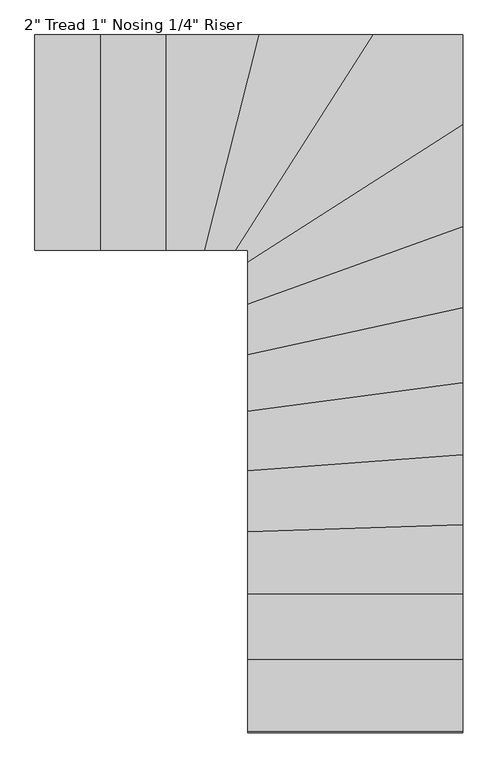
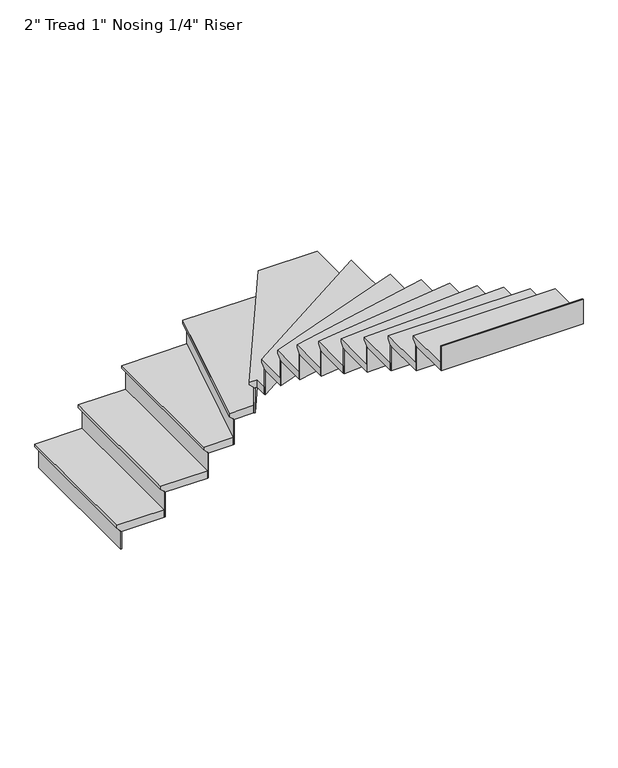
"""IFC4 building model written with IfcOpenShell, lengths in millimetres: stair flight geometry."""

from ifc_helpers import new_model, si_unit, origin, place, context, project, spatial, faceted_brep, source, transform, mapped, element, save


def stair_flight_d6903057(model_context):
    return source(origin(), model_context, "Body", "Brep", [
        faceted_brep([(-12520.2436952, 5104.5187882, 827.6166667), (-12520.2436952, 5104.5187882, 846.6666667), (-12520.2436952, 6018.9187882, 846.6666667), (-12520.2436952, 6018.9187882, 827.6166667), (-12494.8436952, 5104.5187882, 802.2166667), (-12494.8436952, 6018.9187882, 802.2166667), (-12215.4436952, 5104.5187882, 846.6666667), (-12215.4436952, 6018.9187882, 846.6666667), (-12494.8436952, 6018.9187882, 795.8666667), (-12215.4436952, 6018.9187882, 795.8666667), (-12215.4436952, 5104.5187882, 795.8666667), (-12494.8436952, 5104.5187882, 795.8666667)], [[[0, 1, 2, 3]], [[4, 0, 3, 5]], [[2, 1, 6, 7]], [[8, 9, 10, 11]], [[2, 7, 9, 8, 5, 3]], [[8, 11, 4, 5]], [[6, 1, 0, 4, 11, 10]], [[7, 6, 10, 9]]]),
        faceted_brep([(-12494.8436952, 5104.5187882, 795.8666667), (-12494.8436952, 5104.5187882, 677.3333333), (-12488.4936952, 5104.5187882, 677.3333333), (-12488.4936952, 5104.5187882, 795.8666667), (-12494.8436952, 6018.9187882, 795.8666667), (-12488.4936952, 6018.9187882, 795.8666667), (-12488.4936952, 6018.9187882, 677.3333333), (-12494.8436952, 6018.9187882, 677.3333333)], [[[0, 1, 2, 3]], [[4, 5, 6, 7]], [[1, 0, 4, 7]], [[2, 1, 7, 6]], [[3, 2, 6, 5]], [[0, 3, 5, 4]]]),
        faceted_brep([(-12215.4436952, 5104.5187882, 965.2), (-12215.4436952, 5104.5187882, 795.8666667), (-12209.0936952, 5104.5187882, 795.8666667), (-12209.0936952, 5104.5187882, 965.2), (-12215.4436952, 6018.9187882, 965.2), (-12209.0936952, 6018.9187882, 965.2), (-12209.0936952, 6018.9187882, 795.8666667), (-12215.4436952, 6018.9187882, 795.8666667)], [[[0, 1, 2, 3]], [[4, 5, 6, 7]], [[1, 0, 4, 7]], [[2, 1, 7, 6]], [[3, 2, 6, 5]], [[0, 3, 5, 4]]]),
        faceted_brep([(-12240.8436952, 6018.9187882, 1016.0), (-12240.8436952, 5104.5187882, 1016.0), (-11936.0436952, 5104.5187882, 1016.0), (-11936.0436952, 6018.9187882, 1016.0), (-12215.4436952, 6018.9187882, 965.2), (-11936.0436952, 6018.9187882, 965.2), (-11936.0436952, 5104.5187882, 965.2), (-12215.4436952, 5104.5187882, 965.2), (-12215.4436952, 6018.9187882, 971.55), (-12240.8436952, 6018.9187882, 996.95), (-12215.4436952, 5104.5187882, 971.55), (-12240.8436952, 5104.5187882, 996.95)], [[[0, 1, 2, 3]], [[4, 5, 6, 7]], [[0, 3, 5, 4, 8, 9]], [[4, 7, 10, 8]], [[2, 1, 11, 10, 7, 6]], [[3, 2, 6, 5]], [[11, 1, 0, 9]], [[10, 11, 9, 8]]]),
        faceted_brep([(-11936.0436952, 5104.5187882, 1134.5333333), (-11936.0436952, 5104.5187882, 965.2), (-11929.6936952, 5104.5187882, 965.2), (-11929.6936952, 5104.5187882, 1134.5333333), (-11936.0436952, 6018.9187882, 1134.5333333), (-11929.6936952, 6018.9187882, 1134.5333333), (-11929.6936952, 6018.9187882, 965.2), (-11936.0436952, 6018.9187882, 965.2)], [[[0, 1, 2, 3]], [[4, 5, 6, 7]], [[1, 0, 4, 7]], [[2, 1, 7, 6]], [[3, 2, 6, 5]], [[0, 3, 5, 4]]]),
        faceted_brep([(-11961.4436952, 6018.9187882, 1185.3333333), (-11961.4436952, 5104.5187882, 1185.3333333), (-11771.3386614, 5104.5187882, 1185.3333333), (-11540.3529848, 6018.9187882, 1185.3333333), (-11936.0436952, 6018.9187882, 1134.5333333), (-11540.3529848, 6018.9187882, 1134.5333333), (-11771.3386614, 5104.5187882, 1134.5333333), (-11936.0436952, 5104.5187882, 1134.5333333), (-11936.0436952, 6018.9187882, 1140.8833333), (-11961.4436952, 6018.9187882, 1166.2833333), (-11936.0436952, 5104.5187882, 1140.8833333), (-11961.4436952, 5104.5187882, 1166.2833333)], [[[0, 1, 2, 3]], [[4, 5, 6, 7]], [[0, 3, 5, 4, 8, 9]], [[4, 7, 10, 8]], [[2, 1, 11, 10, 7, 6]], [[3, 2, 6, 5]], [[11, 1, 0, 9]], [[10, 11, 9, 8]]]),
        faceted_brep([(-11771.3386614, 5104.5187882, 1303.8666667), (-11771.3386614, 5104.5187882, 1134.5333333), (-11764.7891933, 5104.5187882, 1134.5333333), (-11764.7891933, 5104.5187882, 1303.8666667), (-11540.3529848, 6018.9187882, 1303.8666667), (-11533.8035167, 6018.9187882, 1303.8666667), (-11533.8035167, 6018.9187882, 1134.5333333), (-11540.3529848, 6018.9187882, 1134.5333333)], [[[0, 1, 2, 3]], [[4, 5, 6, 7]], [[1, 0, 4, 7]], [[2, 1, 7, 6]], [[3, 2, 6, 5]], [[0, 3, 5, 4]]]),
        faceted_brep([(-11566.5508569, 6018.9187882, 1354.6666667), (-11797.5365335, 5104.5187882, 1354.6666667), (-11637.0710723, 5104.5187882, 1354.6666667), (-11052.4716369, 6018.9187882, 1354.6666667), (-11540.3529848, 6018.9187882, 1303.8666667), (-11052.4716369, 6018.9187882, 1303.8666667), (-11637.0710723, 5104.5187882, 1303.8666667), (-11771.3386614, 5104.5187882, 1303.8666667), (-11540.3529848, 6018.9187882, 1310.2166667), (-11566.5508569, 6018.9187882, 1335.6166667), (-11771.3386614, 5104.5187882, 1310.2166667), (-11797.5365335, 5104.5187882, 1335.6166667)], [[[0, 1, 2, 3]], [[4, 5, 6, 7]], [[0, 3, 5, 4, 8, 9]], [[4, 7, 10, 8]], [[2, 1, 11, 10, 7, 6]], [[3, 2, 6, 5]], [[11, 1, 0, 9]], [[10, 11, 9, 8]]]),
        faceted_brep([(-11637.0710723, 5104.5187882, 1473.2), (-11637.0710723, 5104.5187882, 1303.8666667), (-11629.5342419, 5104.5187882, 1303.8666667), (-11629.5342419, 5104.5187882, 1473.2), (-11052.4716369, 6018.9187882, 1473.2), (-11044.9348065, 6018.9187882, 1473.2), (-11044.9348065, 6018.9187882, 1303.8666667), (-11052.4716369, 6018.9187882, 1303.8666667)], [[[0, 1, 2, 3]], [[4, 5, 6, 7]], [[1, 0, 4, 7]], [[2, 1, 7, 6]], [[3, 2, 6, 5]], [[0, 3, 5, 4]]]),
        faceted_brep([(-10701.9067057, 5608.0592137, 1524.0), (-10701.9067057, 6018.9187882, 1524.0), (-11082.6189586, 6018.9187882, 1524.0), (-11667.218394, 5104.5187882, 1524.0), (-11616.3067057, 5104.5187882, 1524.0), (-11616.3067057, 5023.4597783, 1524.0), (-10701.9067057, 6018.9187882, 1473.2), (-10701.9067057, 5608.0592137, 1473.2), (-11616.3067057, 5023.4597783, 1473.2), (-11616.3067057, 5104.5187882, 1473.2), (-11637.0710723, 5104.5187882, 1473.2), (-11052.4716369, 6018.9187882, 1473.2), (-11637.0710723, 5104.5187882, 1479.55), (-11052.4716369, 6018.9187882, 1479.55), (-11667.218394, 5104.5187882, 1504.95), (-11082.6189586, 6018.9187882, 1504.95)], [[[0, 1, 2, 3, 4, 5]], [[6, 7, 8, 9, 10, 11]], [[1, 0, 7, 6]], [[11, 10, 12, 13]], [[4, 3, 14, 12, 10, 9]], [[0, 5, 8, 7]], [[14, 3, 2, 15]], [[12, 14, 15, 13]], [[2, 1, 6, 11, 13, 15]], [[5, 4, 9, 8]]]),
        faceted_brep([(-11616.3067057, 5023.4597783, 1642.5333333), (-11616.3067057, 5023.4597783, 1473.2), (-11616.3067057, 5015.9229479, 1473.2), (-11616.3067057, 5015.9229479, 1642.5333333), (-10701.9067057, 5608.0592137, 1642.5333333), (-10701.9067057, 5600.5223833, 1642.5333333), (-10701.9067057, 5600.5223833, 1473.2), (-10701.9067057, 5608.0592137, 1473.2)], [[[0, 1, 2, 3]], [[4, 5, 6, 7]], [[1, 0, 4, 7]], [[2, 1, 7, 6]], [[3, 2, 6, 5]], [[0, 3, 5, 4]]]),
        faceted_brep([(-10701.9067057, 5638.2065353, 1693.3333333), (-11616.3067057, 5053.6070999, 1693.3333333), (-11616.3067057, 4847.5034664, 1693.3333333), (-10701.9067057, 5176.0799712, 1693.3333333), (-10701.9067057, 5608.0592137, 1642.5333333), (-10701.9067057, 5176.0799712, 1642.5333333), (-11616.3067057, 4847.5034664, 1642.5333333), (-11616.3067057, 5023.4597783, 1642.5333333), (-10701.9067057, 5608.0592137, 1648.8833333), (-10701.9067057, 5638.2065353, 1674.2833333), (-11616.3067057, 5023.4597783, 1648.8833333), (-11616.3067057, 5053.6070999, 1674.2833333)], [[[0, 1, 2, 3]], [[4, 5, 6, 7]], [[0, 3, 5, 4, 8, 9]], [[4, 7, 10, 8]], [[2, 1, 11, 10, 7, 6]], [[3, 2, 6, 5]], [[11, 1, 0, 9]], [[10, 11, 9, 8]]]),
        faceted_brep([(-11616.3067057, 4847.5034664, 1811.8666667), (-11616.3067057, 4847.5034664, 1642.5333333), (-11616.3067057, 4840.7559464, 1642.5333333), (-11616.3067057, 4840.7559464, 1811.8666667), (-10701.9067057, 5176.0799712, 1811.8666667), (-10701.9067057, 5169.3324512, 1811.8666667), (-10701.9067057, 5169.3324512, 1642.5333333), (-10701.9067057, 5176.0799712, 1642.5333333)], [[[0, 1, 2, 3]], [[4, 5, 6, 7]], [[1, 0, 4, 7]], [[2, 1, 7, 6]], [[3, 2, 6, 5]], [[0, 3, 5, 4]]]),
        faceted_brep([(-10701.9067057, 5203.0700511, 1862.6666667), (-11616.3067057, 4874.4935463, 1862.6666667), (-11616.3067057, 4633.3870673, 1862.6666667), (-10701.9067057, 4833.3757339, 1862.6666667), (-10701.9067057, 5176.0799712, 1811.8666667), (-10701.9067057, 4833.3757339, 1811.8666667), (-11616.3067057, 4633.3870673, 1811.8666667), (-11616.3067057, 4847.5034664, 1811.8666667), (-10701.9067057, 5176.0799712, 1818.2166667), (-10701.9067057, 5203.0700511, 1843.6166667), (-11616.3067057, 4847.5034664, 1818.2166667), (-11616.3067057, 4874.4935463, 1843.6166667)], [[[0, 1, 2, 3]], [[4, 5, 6, 7]], [[0, 3, 5, 4, 8, 9]], [[4, 7, 10, 8]], [[2, 1, 11, 10, 7, 6]], [[3, 2, 6, 5]], [[11, 1, 0, 9]], [[10, 11, 9, 8]]]),
        faceted_brep([(-11616.3067057, 4633.3870673, 1981.2), (-11616.3067057, 4633.3870673, 1811.8666667), (-11616.3067057, 4626.8869678, 1811.8666667), (-11616.3067057, 4626.8869678, 1981.2), (-10701.9067057, 4833.3757339, 1981.2), (-10701.9067057, 4826.8756344, 1981.2), (-10701.9067057, 4826.8756344, 1811.8666667), (-10701.9067057, 4833.3757339, 1811.8666667)], [[[0, 1, 2, 3]], [[4, 5, 6, 7]], [[1, 0, 4, 7]], [[2, 1, 7, 6]], [[3, 2, 6, 5]], [[0, 3, 5, 4]]]),
        faceted_brep([(-10701.9067057, 4859.376132, 2032.0), (-11616.3067057, 4659.3874654, 2032.0), (-11616.3067057, 4393.8400272, 2032.0), (-10701.9067057, 4514.8804393, 2032.0), (-10701.9067057, 4833.3757339, 1981.2), (-10701.9067057, 4514.8804393, 1981.2), (-11616.3067057, 4393.8400272, 1981.2), (-11616.3067057, 4633.3870673, 1981.2), (-10701.9067057, 4833.3757339, 1987.55), (-10701.9067057, 4859.376132, 2012.95), (-11616.3067057, 4633.3870673, 1987.55), (-11616.3067057, 4659.3874654, 2012.95)], [[[0, 1, 2, 3]], [[4, 5, 6, 7]], [[0, 3, 5, 4, 8, 9]], [[4, 7, 10, 8]], [[2, 1, 11, 10, 7, 6]], [[3, 2, 6, 5]], [[11, 1, 0, 9]], [[10, 11, 9, 8]]]),
        faceted_brep([(-11616.3067057, 4393.8400272, 2150.5333333), (-11616.3067057, 4393.8400272, 1981.2), (-11616.3067057, 4387.4346359, 1981.2), (-11616.3067057, 4387.4346359, 2150.5333333), (-10701.9067057, 4514.8804393, 2150.5333333), (-10701.9067057, 4508.4750479, 2150.5333333), (-10701.9067057, 4508.4750479, 1981.2), (-10701.9067057, 4514.8804393, 1981.2)], [[[0, 1, 2, 3]], [[4, 5, 6, 7]], [[1, 0, 4, 7]], [[2, 1, 7, 6]], [[3, 2, 6, 5]], [[0, 3, 5, 4]]]),
        faceted_brep([(-10701.9067057, 4540.5020047, 2201.3333333), (-11616.3067057, 4419.4615927, 2201.3333333), (-11616.3067057, 4141.2933024, 2201.3333333), (-10701.9067057, 4208.9315067, 2201.3333333), (-10701.9067057, 4514.8804393, 2150.5333333), (-10701.9067057, 4208.9315067, 2150.5333333), (-11616.3067057, 4141.2933024, 2150.5333333), (-11616.3067057, 4393.8400272, 2150.5333333), (-10701.9067057, 4514.8804393, 2156.8833333), (-10701.9067057, 4540.5020047, 2182.2833333), (-11616.3067057, 4393.8400272, 2156.8833333), (-11616.3067057, 4419.4615927, 2182.2833333)], [[[0, 1, 2, 3]], [[4, 5, 6, 7]], [[0, 3, 5, 4, 8, 9]], [[4, 7, 10, 8]], [[2, 1, 11, 10, 7, 6]], [[3, 2, 6, 5]], [[11, 1, 0, 9]], [[10, 11, 9, 8]]]),
        faceted_brep([(-11616.3067057, 4141.2933024, 2319.8666667), (-11616.3067057, 4141.2933024, 2150.5333333), (-11616.3067057, 4134.9259539, 2150.5333333), (-11616.3067057, 4134.9259539, 2319.8666667), (-10701.9067057, 4208.9315067, 2319.8666667), (-10701.9067057, 4202.5641582, 2319.8666667), (-10701.9067057, 4202.5641582, 2150.5333333), (-10701.9067057, 4208.9315067, 2150.5333333)], [[[0, 1, 2, 3]], [[4, 5, 6, 7]], [[1, 0, 4, 7]], [[2, 1, 7, 6]], [[3, 2, 6, 5]], [[0, 3, 5, 4]]]),
        faceted_brep([(-10701.9067057, 4234.4009008, 2370.6666667), (-11616.3067057, 4166.7626966, 2370.6666667), (-11616.3067057, 3881.2141892, 2370.6666667), (-10701.9067057, 3910.3236734, 2370.6666667), (-10701.9067057, 4208.9315067, 2319.8666667), (-10701.9067057, 3910.3236734, 2319.8666667), (-11616.3067057, 3881.2141892, 2319.8666667), (-11616.3067057, 4141.2933024, 2319.8666667), (-10701.9067057, 4208.9315067, 2326.2166667), (-10701.9067057, 4234.4009008, 2351.6166667), (-11616.3067057, 4141.2933024, 2326.2166667), (-11616.3067057, 4166.7626966, 2351.6166667)], [[[0, 1, 2, 3]], [[4, 5, 6, 7]], [[0, 3, 5, 4, 8, 9]], [[4, 7, 10, 8]], [[2, 1, 11, 10, 7, 6]], [[3, 2, 6, 5]], [[11, 1, 0, 9]], [[10, 11, 9, 8]]]),
        faceted_brep([(-11616.3067057, 3881.2141892, 2489.2), (-11616.3067057, 3881.2141892, 2319.8666667), (-11616.3067057, 3874.8609724, 2319.8666667), (-11616.3067057, 3874.8609724, 2489.2), (-10701.9067057, 3910.3236734, 2489.2), (-10701.9067057, 3903.9704565, 2489.2), (-10701.9067057, 3903.9704565, 2319.8666667), (-10701.9067057, 3910.3236734, 2319.8666667)], [[[0, 1, 2, 3]], [[4, 5, 6, 7]], [[1, 0, 4, 7]], [[2, 1, 7, 6]], [[3, 2, 6, 5]], [[0, 3, 5, 4]]]),
        faceted_brep([(-10701.9067057, 3935.7365407, 2540.0), (-11616.3067057, 3906.6270566, 2540.0), (-11616.3067057, 3616.3817987, 2540.0), (-10701.9067057, 3616.3817987, 2540.0), (-10701.9067057, 3910.3236734, 2489.2), (-10701.9067057, 3616.3817987, 2489.2), (-11616.3067057, 3616.3817987, 2489.2), (-11616.3067057, 3881.2141892, 2489.2), (-10701.9067057, 3910.3236734, 2495.55), (-10701.9067057, 3935.7365407, 2520.95), (-11616.3067057, 3881.2141892, 2495.55), (-11616.3067057, 3906.6270566, 2520.95)], [[[0, 1, 2, 3]], [[4, 5, 6, 7]], [[0, 3, 5, 4, 8, 9]], [[4, 7, 10, 8]], [[2, 1, 11, 10, 7, 6]], [[3, 2, 6, 5]], [[11, 1, 0, 9]], [[10, 11, 9, 8]]]),
        faceted_brep([(-11616.3067057, 3616.3817987, 2658.5333333), (-11616.3067057, 3616.3817987, 2489.2), (-11616.3067057, 3610.0317987, 2489.2), (-11616.3067057, 3610.0317987, 2658.5333333), (-10701.9067057, 3616.3817987, 2658.5333333), (-10701.9067057, 3610.0317987, 2658.5333333), (-10701.9067057, 3610.0317987, 2489.2), (-10701.9067057, 3616.3817987, 2489.2)], [[[0, 1, 2, 3]], [[4, 5, 6, 7]], [[1, 0, 4, 7]], [[2, 1, 7, 6]], [[3, 2, 6, 5]], [[0, 3, 5, 4]]]),
        faceted_brep([(-10701.9067057, 3641.7817987, 2709.3333333), (-11616.3067057, 3641.7817987, 2709.3333333), (-11616.3067057, 3336.9817987, 2709.3333333), (-10701.9067057, 3336.9817987, 2709.3333333), (-10701.9067057, 3616.3817987, 2658.5333333), (-10701.9067057, 3336.9817987, 2658.5333333), (-11616.3067057, 3336.9817987, 2658.5333333), (-11616.3067057, 3616.3817987, 2658.5333333), (-10701.9067057, 3616.3817987, 2664.8833333), (-10701.9067057, 3641.7817987, 2690.2833333), (-11616.3067057, 3616.3817987, 2664.8833333), (-11616.3067057, 3641.7817987, 2690.2833333)], [[[0, 1, 2, 3]], [[4, 5, 6, 7]], [[0, 3, 5, 4, 8, 9]], [[4, 7, 10, 8]], [[2, 1, 11, 10, 7, 6]], [[3, 2, 6, 5]], [[11, 1, 0, 9]], [[10, 11, 9, 8]]]),
        faceted_brep([(-11616.3067057, 3336.9817987, 2827.8666667), (-11616.3067057, 3336.9817987, 2658.5333333), (-11616.3067057, 3330.6317987, 2658.5333333), (-11616.3067057, 3330.6317987, 2827.8666667), (-10701.9067057, 3336.9817987, 2827.8666667), (-10701.9067057, 3330.6317987, 2827.8666667), (-10701.9067057, 3330.6317987, 2658.5333333), (-10701.9067057, 3336.9817987, 2658.5333333)], [[[0, 1, 2, 3]], [[4, 5, 6, 7]], [[1, 0, 4, 7]], [[2, 1, 7, 6]], [[3, 2, 6, 5]], [[0, 3, 5, 4]]]),
        faceted_brep([(-11616.3067057, 3057.5817987, 2997.2), (-11616.3067057, 3057.5817987, 2827.8666667), (-11616.3067057, 3051.2317987, 2827.8666667), (-11616.3067057, 3051.2317987, 2997.2), (-10701.9067057, 3057.5817987, 2997.2), (-10701.9067057, 3051.2317987, 2997.2), (-10701.9067057, 3051.2317987, 2827.8666667), (-10701.9067057, 3057.5817987, 2827.8666667)], [[[0, 1, 2, 3]], [[4, 5, 6, 7]], [[1, 0, 4, 7]], [[2, 1, 7, 6]], [[3, 2, 6, 5]], [[0, 3, 5, 4]]]),
        faceted_brep([(-10701.9067057, 3362.3817987, 2878.6666667), (-11616.3067057, 3362.3817987, 2878.6666667), (-11616.3067057, 3057.5817987, 2878.6666667), (-10701.9067057, 3057.5817987, 2878.6666667), (-10701.9067057, 3336.9817987, 2827.8666667), (-10701.9067057, 3057.5817987, 2827.8666667), (-11616.3067057, 3057.5817987, 2827.8666667), (-11616.3067057, 3336.9817987, 2827.8666667), (-10701.9067057, 3336.9817987, 2834.2166667), (-10701.9067057, 3362.3817987, 2859.6166667), (-11616.3067057, 3336.9817987, 2834.2166667), (-11616.3067057, 3362.3817987, 2859.6166667)], [[[0, 1, 2, 3]], [[4, 5, 6, 7]], [[0, 3, 5, 4, 8, 9]], [[4, 7, 10, 8]], [[2, 1, 11, 10, 7, 6]], [[3, 2, 6, 5]], [[11, 1, 0, 9]], [[10, 11, 9, 8]]]),
    ])


if __name__ == "__main__":
    model = new_model("IFC4")
    model_context = context("Model", 3, world=origin())
    ifc_project = project(units=[si_unit("LENGTHUNIT", "METRE", prefix="MILLI")], contexts=[model_context])
    site = spatial("IfcSite", under=ifc_project)
    building = spatial("IfcBuilding", under=site)
    placement = place(None, origin())
    stair_flight_shape = stair_flight_d6903057(model_context)
    element("IfcStairFlight", 1, ObjectType="2\" Tread 1\" Nosing 1/4\" Riser", at=placement, inside=building, context=model_context, shape_type="MappedRepresentation", body=[
        mapped(stair_flight_shape, transform((0.0, 0.0, 0.0), x_axis=(1.0, 0.0, 0.0), y_axis=(0.0, 1.0, 0.0), z_axis=(0.0, 0.0, 1.0))),
    ])
    save(model, "model.ifc")
